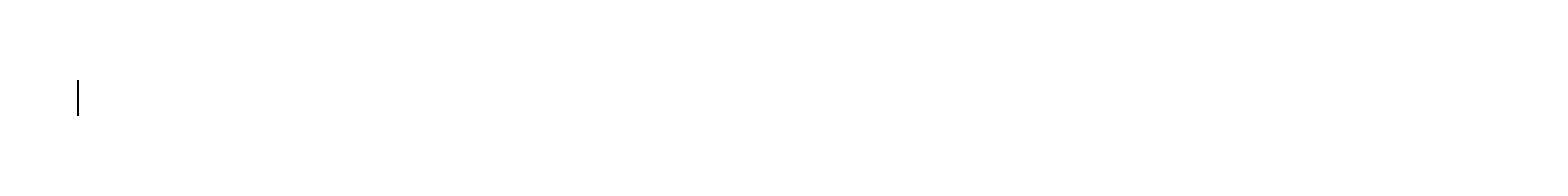
# Model space of a CAD drawing. Units: inches. Extents: x 35362 to 73946, y 43607 to 67532.
# Tile 102 of 134: x 50119 to 50761, y 49320 to 49328. Entities that reach past the tile are written whole.
import ezdxf

# ---------------------------------------------------------------- set-up
doc = ezdxf.new("R2010")
doc.units = ezdxf.units.IN
doc.header["$MEASUREMENT"] = 0
doc.layers.add('A-ANNO-DIMS', color=2, linetype='Continuous', lineweight=18)
doc.styles.get("Standard").update_dxf_attribs({"font": 'arial.ttf'})
doc.dimstyles.get("Standard").update_dxf_attribs({"dimtxt": 0.18, "dimasz": 0.18, "dimexe": 0.18, "dimexo": 0.0625, "dimgap": 0.09, "dimtad": 0, "dimtih": 1, "dimtoh": 1, "dimdec": 4, "dimzin": 0, "dimdsep": 46, "dimtxsty": 'Standard', "dimcen": 0.09, "dimadec": 0, "dimazin": 0, "dimtfac": 1, "dimtdec": 4, "dimtofl": 0, "dimtmove": 0, "dimatfit": 3, "dimfxl": 1, "dimtolj": 1, "dimtzin": 0, "dimarcsym": 0})

# ---------------------------------------------------------------- blocks, each defined once
blk = doc.blocks.new('*D11')
at = {"layer": 'A-ANNO-DIMS', "color": 0, "lineweight": -2, "transparency": 16777216}
for p, q in [((47978.66, 56028.77), (47978.66, 43606.68)), ((53109.76, 56028.77), (53109.76, 43606.68)), ((47978.84, 43606.86), (50543.87, 43606.86)), ((53109.58, 43606.86), (50544.55, 43606.86))]:
    blk.add_line(p, q, dxfattribs=at)
at = {"layer": 'A-ANNO-DIMS', "color": 0, "transparency": 16777216}
for points in [[(47978.84, 43606.89), (47978.84, 43606.83), (47978.66, 43606.86)], [(53109.58, 43606.89), (53109.58, 43606.83), (53109.76, 43606.86)]]:
    blk.add_solid(points, dxfattribs=at)
at = {"layer": 'Defpoints', "color": 0, "transparency": 16777216}
for p in [(47978.66, 56028.84), (53109.76, 56028.84), (53109.76, 43606.86)]:
    blk.add_point(p, dxfattribs=at)
at = {"layer": 'A-ANNO-DIMS', "color": 0, "transparency": 16777216, "insert": (50544.21, 43606.86), "char_height": 0.18, "attachment_point": 5}
blk.add_mtext('\\A1;5131', dxfattribs=at)
blk = doc.blocks.new('*D13')
at = {"layer": 'A-ANNO-DIMS', "color": 0, "lineweight": -2, "transparency": 16777216}
for p, q in [((48373.49, 51694.02), (48373.49, 43606.68)), ((51029.04, 51694.02), (51029.04, 43606.68)), ((48373.67, 43606.86), (49700.8, 43606.86)), ((51028.86, 43606.86), (49701.73, 43606.86))]:
    blk.add_line(p, q, dxfattribs=at)
at = {"layer": 'A-ANNO-DIMS', "color": 0, "transparency": 16777216}
for points in [[(48373.67, 43606.89), (48373.67, 43606.83), (48373.49, 43606.86)], [(51028.86, 43606.89), (51028.86, 43606.83), (51029.04, 43606.86)]]:
    blk.add_solid(points, dxfattribs=at)
at = {"layer": 'Defpoints', "color": 0, "transparency": 16777216}
for p in [(48373.49, 51694.09), (51029.04, 51694.09), (51029.04, 43606.86)]:
    blk.add_point(p, dxfattribs=at)
at = {"layer": 'A-ANNO-DIMS', "color": 0, "transparency": 16777216, "insert": (49701.27, 43606.86), "char_height": 0.18, "attachment_point": 5}
blk.add_mtext('\\A1;2655.6', dxfattribs=at)
blk = doc.blocks.new('*D17')
at = {"layer": 'A-ANNO-DIMS', "color": 0, "lineweight": -2, "transparency": 16777216}
for p, q in [((49923.31, 61293.22), (49923.31, 43606.68)), ((51913.93, 61293.22), (51913.93, 43606.68)), ((49923.49, 43606.86), (50918.16, 43606.86)), ((51913.75, 43606.86), (50919.07, 43606.86))]:
    blk.add_line(p, q, dxfattribs=at)
at = {"layer": 'A-ANNO-DIMS', "color": 0, "transparency": 16777216}
for points in [[(49923.49, 43606.89), (49923.49, 43606.83), (49923.31, 43606.86)], [(51913.75, 43606.89), (51913.75, 43606.83), (51913.93, 43606.86)]]:
    blk.add_solid(points, dxfattribs=at)
at = {"layer": 'Defpoints', "color": 0, "transparency": 16777216}
for p in [(49923.31, 61293.29), (51913.93, 61293.29), (51913.93, 43606.86)]:
    blk.add_point(p, dxfattribs=at)
at = {"layer": 'A-ANNO-DIMS', "color": 0, "transparency": 16777216, "insert": (50918.62, 43606.86), "char_height": 0.18, "attachment_point": 5}
blk.add_mtext('\\A1;1990.6', dxfattribs=at)
blk = doc.blocks.new('*D40')
at = {"layer": 'A-ANNO-DIMS', "color": 0, "lineweight": -2, "transparency": 16777216}
for p, q in [((56873.54, 53351.53), (35361.77, 53351.53)), ((35361.95, 53351.35), (35361.95, 51333.28)), ((35361.95, 49314.85), (35361.95, 51332.92)), ((51806.45, 49314.67), (35361.77, 49314.67))]:
    blk.add_line(p, q, dxfattribs=at)
at = {"layer": 'A-ANNO-DIMS', "color": 0, "transparency": 16777216}
for points in [[(35361.92, 53351.35), (35361.98, 53351.35), (35361.95, 53351.53)], [(35361.92, 49314.85), (35361.98, 49314.85), (35361.95, 49314.67)]]:
    blk.add_solid(points, dxfattribs=at)
at = {"layer": 'Defpoints', "color": 0, "transparency": 16777216}
for p in [(35361.95, 53351.53), (56873.6, 53351.53), (51806.52, 49314.67)]:
    blk.add_point(p, dxfattribs=at)
at = {"layer": 'A-ANNO-DIMS', "color": 0, "transparency": 16777216, "insert": (35361.95, 51333.1), "char_height": 0.18, "attachment_point": 5}
blk.add_mtext('\\A1;4036.9', dxfattribs=at)
blk = doc.blocks.new('*D67')
at = {"layer": 'A-ANNO-DIMS', "color": 0, "lineweight": -2, "transparency": 16777216}
for p, q in [((56873.54, 53351.53), (35361.77, 53351.53)), ((35361.95, 53351.35), (35361.95, 49400.89)), ((35361.95, 45450.07), (35361.95, 49400.53)), ((53793.58, 45449.89), (35361.77, 45449.89))]:
    blk.add_line(p, q, dxfattribs=at)
at = {"layer": 'A-ANNO-DIMS', "color": 0, "transparency": 16777216}
for points in [[(35361.92, 53351.35), (35361.98, 53351.35), (35361.95, 53351.53)], [(35361.92, 45450.07), (35361.98, 45450.07), (35361.95, 45449.89)]]:
    blk.add_solid(points, dxfattribs=at)
at = {"layer": 'Defpoints', "color": 0, "transparency": 16777216}
for p in [(35361.95, 53351.53), (56873.6, 53351.53), (53793.64, 45449.89)]:
    blk.add_point(p, dxfattribs=at)
at = {"layer": 'A-ANNO-DIMS', "color": 0, "transparency": 16777216, "insert": (35361.95, 49400.71), "char_height": 0.18, "attachment_point": 5}
blk.add_mtext('\\A1;7901.6', dxfattribs=at)
blk = doc.blocks.new('*D107')
at = {"layer": 'A-ANNO-DIMS', "color": 0, "lineweight": -2, "transparency": 16777216}
for p, q in [((50139.56, 59850.01), (50139.56, 43606.68)), ((51320.81, 59850.01), (51320.81, 43606.68)), ((50139.74, 43606.86), (50729.73, 43606.86)), ((51320.63, 43606.86), (50730.64, 43606.86))]:
    blk.add_line(p, q, dxfattribs=at)
at = {"layer": 'A-ANNO-DIMS', "color": 0, "transparency": 16777216}
for points in [[(50139.74, 43606.89), (50139.74, 43606.83), (50139.56, 43606.86)], [(51320.63, 43606.89), (51320.63, 43606.83), (51320.81, 43606.86)]]:
    blk.add_solid(points, dxfattribs=at)
at = {"layer": 'Defpoints', "color": 0, "transparency": 16777216}
for p in [(50139.56, 59850.08), (51320.81, 59850.08), (51320.81, 43606.86)]:
    blk.add_point(p, dxfattribs=at)
at = {"layer": 'A-ANNO-DIMS', "color": 0, "transparency": 16777216, "insert": (50730.19, 43606.86), "char_height": 0.18, "attachment_point": 5}
blk.add_mtext('\\A1;1181.3', dxfattribs=at)

msp = doc.modelspace()

# ---------------------------------------------------------------- dimensions: what is measured, and where the dimension line sits
at = {"layer": 'A-ANNO-DIMS'}
for base, p1, p2, override, picture, middle in [((51913.931, 43606.859), (49923.307, 61293.286), (51913.931, 61293.286), {"dimdec": 1, "dimlfac": 1, "dimrnd": 0, "dimzin": 0, "dimdsep": 46, "dimlunit": 2}, '*D17', (50918.619, 43606.859)), ((51320.8133, 43606.859), (50139.5627, 59850.0769), (51320.8133, 59850.0769), {"dimdec": 1, "dimlfac": 1, "dimrnd": 0, "dimzin": 0, "dimdsep": 46, "dimlunit": 2}, '*D107', (50730.188, 43606.859)), ((53109.76, 43606.859), (47978.665, 56028.836), (53109.76, 56028.836), {"dimdec": 0, "dimlfac": 1, "dimrnd": 0, "dimzin": 0, "dimdsep": 46, "dimlunit": 2}, '*D11', (50544.212, 43606.859)), ((51029.043, 43606.859), (48373.492, 51694.087), (51029.043, 51694.087), {"dimdec": 1, "dimlfac": 1, "dimrnd": 0, "dimzin": 0, "dimdsep": 46, "dimlunit": 2}, '*D13', (49701.267, 43606.859))]:
    dim = msp.add_linear_dim(base=base, p1=p1, p2=p2, dimstyle='Standard', override=override, dxfattribs=at)
    dim.commit()
    dim.dimension.update_dxf_attribs({"geometry": picture, "text_midpoint": middle})
for p1, picture, middle in [((51806.517, 49314.669), '*D40', (35361.949, 51333.099)), ((53793.638, 45449.894), '*D67', (35361.949, 49400.712))]:
    dim = msp.add_linear_dim(base=(35361.949, 53351.529), p1=p1, p2=(56873.602, 53351.529), angle=90, dimstyle='Standard', override={"dimdec": 1, "dimlfac": 1, "dimrnd": 0, "dimzin": 0, "dimdsep": 46, "dimlunit": 2}, dxfattribs=at)
    dim.commit()
    dim.dimension.update_dxf_attribs({"geometry": picture, "text_midpoint": middle})

doc.saveas('drawing.dxf')
